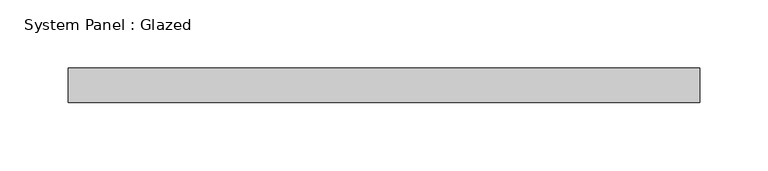
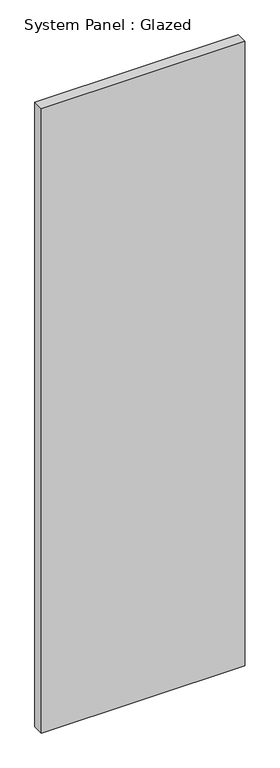
"""IFC4 building model written with IfcOpenShell, lengths in millimetres: plate geometry, System Panel : Glazed."""

from ifc_helpers import new_model, si_unit, origin, origin_with_axes, place, context, project, spatial, polyline, outline, extrude, source, transform, mapped, element, save


def system_panel_glazed_ca6a4ba2(model_context):
    return source(origin(), model_context, "Body", "SweptSolid", [
        extrude(outline(polyline([(231.775, 19.05), (-231.775, 19.05), (-231.775, 44.45), (231.775, 44.45), (231.775, 19.05)])), origin_with_axes(), (0.0, 0.0, 1.0), 1503.931829),
    ])


if __name__ == "__main__":
    model = new_model("IFC4")
    model_context = context("Model", 3, world=origin())
    ifc_project = project(units=[si_unit("LENGTHUNIT", "METRE", prefix="MILLI")], contexts=[model_context])
    site = spatial("IfcSite", under=ifc_project)
    building = spatial("IfcBuilding", under=site)
    placement = place(None, origin())
    system_panel_glazed_shape = system_panel_glazed_ca6a4ba2(model_context)
    element("IfcPlate", 1, ObjectType="System Panel : Glazed", at=placement, inside=building, context=model_context, shape_type="MappedRepresentation", body=[
        mapped(system_panel_glazed_shape, transform((0.0, 0.0, 0.0), x_axis=(1.0, 0.0, 0.0), y_axis=(0.0, 1.0, 0.0), z_axis=(0.0, 0.0, 1.0))),
    ])
    save(model, "model.ifc")

# Revit data of these elements
# Type "System Panel : Glazed"
#   Construction Type Id = "GSP4R"
#   Analytic Construction = "1/8 in Pilkington single glazing"
#   Visual Light Transmittance = 0.9
#   Solar Heat Gain Coefficient = 0.86
#   Heat Transfer Coefficient (U) = 1.18115 BTU/(h·ft²·°F)
#   Define Thermal Properties by = 1
# Element 1 (IfcPlate, "System Panel : Glazed")
#   Materials on its faces: "Glass"
# Materials
#   "Glass": class "Glass", colour RGB 0 128 192, transparency 0.75, Description = "Soda Lime Glass", Cost = 0
